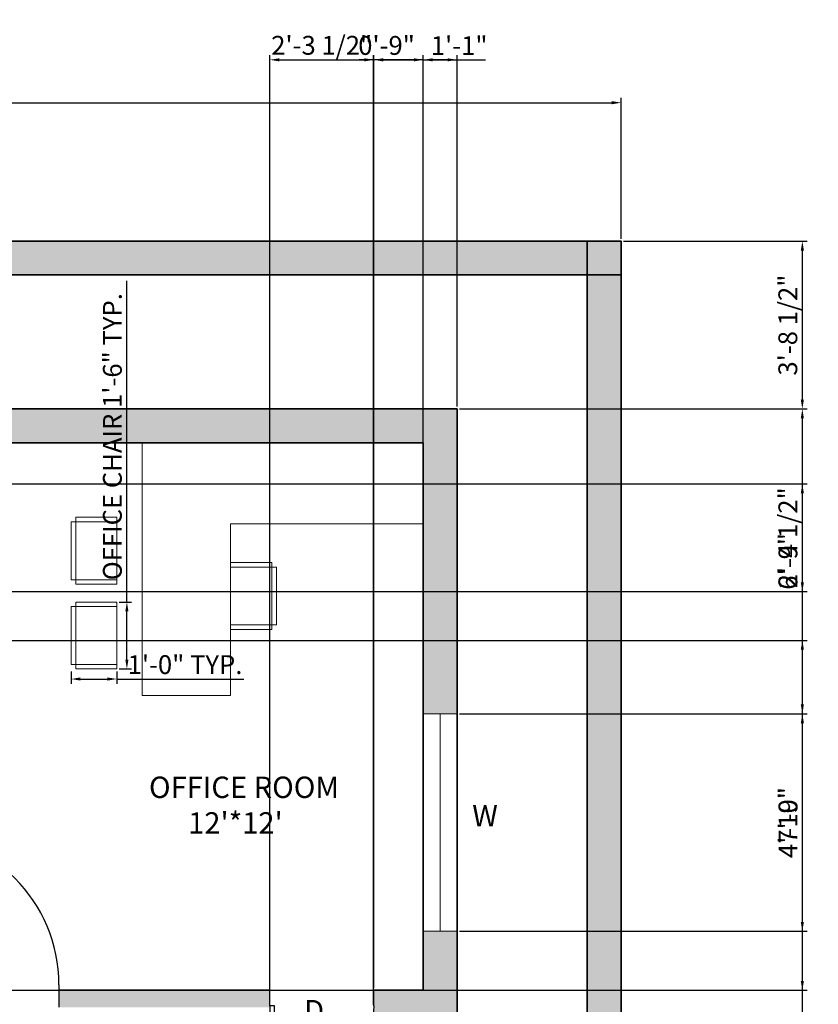
# Model space of a CAD drawing. Units: inches. Extents: x 2130 to 2621, y 981 to 1994.
# Tile 4 of 4: x 2409 to 2621, y 1732 to 1994. Entities that reach past the tile are written whole.
import ezdxf

# ---------------------------------------------------------------- set-up
doc = ezdxf.new("R2010")
doc.units = ezdxf.units.IN
for name, color, linetype, lineweight in [('A-ANNO-DIMS', 2, 'Continuous', 18), ('A-ANNO-TEXT', 10, 'Continuous', 18), ('A-AREA-IDEN', 10, 'Continuous', 18), ('A-WALL-PATT', 140, 'Continuous', 13), ('C-PROP', 7, 'Continuous', 35), ('C-PROP-PATT', 140, 'Continuous', 13), ('DOOR', 130, 'Continuous', 25), ('FUR', 190, 'Continuous', 18), ('WALL', 140, 'Continuous', 35), ('WIND', 210, 'Continuous', 18)]:
    doc.layers.add(name, color=color, linetype=linetype, lineweight=lineweight)
doc.styles.get("Standard").update_dxf_attribs({"font": 'arial.ttf'})
doc.dimstyles.new('ISO-25', dxfattribs={"dimtxt": 5, "dimasz": 2.5, "dimexe": 1.25, "dimexo": 0.625, "dimtad": 1, "dimdec": 0, "dimlunit": 4, "dimtxsty": 'Standard', "dimcen": 2.5, "dimadec": 0, "dimazin": 0, "dimtfac": 1, "dimtdec": 0, "dimtmove": 0, "dimatfit": 3, "dimfxl": 1, "dimarcsym": 0})

# ---------------------------------------------------------------- blocks, each defined once
blk = doc.blocks.new('*U2')
for p, q in [((0, 0), (0, -6)), ((40, 0), (40, -6))]:
    blk.add_line(p, q)
blk.add_lwpolyline([(0, 0), (0, 40), (1.75, 40), (1.75, 0)], close=True)
blk.add_arc((0, 0), 40, 0, 90)
blk = doc.blocks.new('*D9')
at = {"layer": 'A-ANNO-DIMS', "color": 0, "lineweight": -2, "transparency": 16777216}
for p, q in [((2188.76, 1935.64), (2188.76, 1973.06)), ((2568.76, 1935.64), (2568.76, 1973.06)), ((2191.26, 1971.81), (2566.26, 1971.81))]:
    blk.add_line(p, q, dxfattribs=at)
at = {"layer": 'A-ANNO-DIMS', "color": 0, "transparency": 16777216}
for points in [[(2191.26, 1972.23), (2191.26, 1971.39), (2188.76, 1971.81)], [(2566.26, 1972.23), (2566.26, 1971.39), (2568.76, 1971.81)]]:
    blk.add_solid(points, dxfattribs=at)
at = {"layer": 'Defpoints', "color": 0, "transparency": 16777216}
for p in [(2568.76, 1971.81), (2188.76, 1935.02), (2568.76, 1935.02)]:
    blk.add_point(p, dxfattribs=at)
at = {"layer": 'A-ANNO-DIMS', "color": 0, "transparency": 16777216, "insert": (2378.76, 1974.99), "char_height": 5, "attachment_point": 5}
blk.add_mtext('31\'-8"', dxfattribs=at)
blk = doc.blocks.new('CHAIR-OFFICE')
for p, q in [((0, 1.2), (0, 16.6)), ((0, 16.6), (1.25, 16.6)), ((1.25, 16.6), (1.25, 17.78)), ((1.25, 17.78), (12.18, 17.78)), ((12.18, 17.78), (12.18, 16.6)), ((12.18, 0), (12.18, 2.81)), ((1.25, 1.2), (0, 1.2)), ((1.25, 1.2), (1.25, 0)), ((1.25, 0), (12.18, 0))]:
    blk.add_line(p, q)
blk.add_lwpolyline([(12.18, 16.6), (1.25, 16.6), (1.25, 1.2), (12.18, 1.2)], close=True)
blk = doc.blocks.new('*D17')
at = {"layer": 'A-ANNO-DIMS', "color": 0, "lineweight": -2, "transparency": 16777216}
for p, q in [((2437.35, 1839.09), (2437.35, 1924.49)), ((2435.31, 1839.09), (2438.6, 1839.09)), ((2437.35, 1823.81), (2437.35, 1836.59)), ((2435.31, 1821.31), (2438.6, 1821.31))]:
    blk.add_line(p, q, dxfattribs=at)
at = {"layer": 'A-ANNO-DIMS', "color": 0, "transparency": 16777216}
for points in [[(2436.94, 1836.59), (2437.77, 1836.59), (2437.35, 1839.09)], [(2436.94, 1823.81), (2437.77, 1823.81), (2437.35, 1821.31)]]:
    blk.add_solid(points, dxfattribs=at)
at = {"layer": 'Defpoints', "color": 0, "transparency": 16777216}
for p in [(2434.69, 1839.09), (2437.35, 1839.09), (2434.69, 1821.31)]:
    blk.add_point(p, dxfattribs=at)
at = {"layer": 'A-ANNO-DIMS', "color": 0, "transparency": 16777216, "insert": (2434.14, 1883.04), "char_height": 5, "attachment_point": 5, "rotation": 90}
blk.add_mtext('OFFICE CHAIR 1\'-6" TYP.', dxfattribs=at)
blk = doc.blocks.new('*D18')
at = {"layer": 'A-ANNO-DIMS', "color": 0, "lineweight": -2, "transparency": 16777216}
for p, q in [((2422.5, 1820.68), (2422.5, 1817.39)), ((2425, 1818.64), (2432.19, 1818.64)), ((2434.69, 1820.68), (2434.69, 1817.39)), ((2434.69, 1818.64), (2468.44, 1818.64))]:
    blk.add_line(p, q, dxfattribs=at)
at = {"layer": 'A-ANNO-DIMS', "color": 0, "transparency": 16777216}
for points in [[(2425, 1819.06), (2425, 1818.23), (2422.5, 1818.64)], [(2432.19, 1819.06), (2432.19, 1818.23), (2434.69, 1818.64)]]:
    blk.add_solid(points, dxfattribs=at)
at = {"layer": 'Defpoints', "color": 0, "transparency": 16777216}
for p in [(2422.5, 1821.31), (2434.69, 1821.31), (2434.69, 1818.64)]:
    blk.add_point(p, dxfattribs=at)
at = {"layer": 'A-ANNO-DIMS', "color": 0, "transparency": 16777216, "insert": (2452.81, 1821.82), "char_height": 5, "attachment_point": 5}
blk.add_mtext('1\'-0" TYP.', dxfattribs=at)
blk = doc.blocks.new('*D24')
at = {"layer": 'A-ANNO-DIMS', "color": 0, "lineweight": -2, "transparency": 16777216}
for p, q in [((2525.79, 1890.41), (2618.19, 1890.41)), ((2616.94, 1355.91), (2616.94, 1887.91)), ((2525.79, 1353.41), (2618.19, 1353.41))]:
    blk.add_line(p, q, dxfattribs=at)
at = {"layer": 'A-ANNO-DIMS', "color": 0, "transparency": 16777216}
for points in [[(2616.52, 1887.91), (2617.35, 1887.91), (2616.94, 1890.41)], [(2616.52, 1355.91), (2617.35, 1355.91), (2616.94, 1353.41)]]:
    blk.add_solid(points, dxfattribs=at)
at = {"layer": 'Defpoints', "color": 0, "transparency": 16777216}
for p in [(2525.16, 1890.41), (2616.94, 1890.41), (2525.16, 1353.41)]:
    blk.add_point(p, dxfattribs=at)
at = {"layer": 'A-ANNO-DIMS', "color": 0, "transparency": 16777216, "insert": (2613.76, 1621.91), "char_height": 5, "attachment_point": 5, "rotation": 90}
blk.add_mtext('44\'-9"', dxfattribs=at)
blk = doc.blocks.new('*D26')
at = {"layer": 'A-ANNO-DIMS', "color": 0, "lineweight": -2, "transparency": 16777216}
for p, q in [((2569.38, 1935.02), (2618.19, 1935.02)), ((2616.94, 1892.91), (2616.94, 1932.52)), ((2525.79, 1890.41), (2618.19, 1890.41))]:
    blk.add_line(p, q, dxfattribs=at)
at = {"layer": 'A-ANNO-DIMS', "color": 0, "transparency": 16777216}
for points in [[(2616.52, 1932.52), (2617.35, 1932.52), (2616.94, 1935.02)], [(2616.52, 1892.91), (2617.35, 1892.91), (2616.94, 1890.41)]]:
    blk.add_solid(points, dxfattribs=at)
at = {"layer": 'Defpoints', "color": 0, "transparency": 16777216}
for p in [(2568.76, 1935.02), (2616.94, 1935.02), (2525.16, 1890.41)]:
    blk.add_point(p, dxfattribs=at)
at = {"layer": 'A-ANNO-DIMS', "color": 0, "transparency": 16777216, "insert": (2613.72, 1912.71), "char_height": 5, "attachment_point": 5, "rotation": 90}
blk.add_mtext('3\'-8 1/2"', dxfattribs=at)
blk = doc.blocks.new('*D29')
at = {"layer": 'A-ANNO-DIMS', "color": 0, "lineweight": -2, "transparency": 16777216}
for p, q in [((2368.29, 1828.91), (2618.19, 1828.91)), ((2616.94, 1738.41), (2616.94, 1826.41)), ((2368.29, 1735.91), (2618.19, 1735.91))]:
    blk.add_line(p, q, dxfattribs=at)
at = {"layer": 'A-ANNO-DIMS', "color": 0, "transparency": 16777216}
for points in [[(2616.52, 1826.41), (2617.35, 1826.41), (2616.94, 1828.91)], [(2616.52, 1738.41), (2617.35, 1738.41), (2616.94, 1735.91)]]:
    blk.add_solid(points, dxfattribs=at)
at = {"layer": 'Defpoints', "color": 0, "transparency": 16777216}
for p in [(2367.66, 1828.91), (2616.94, 1828.91), (2367.66, 1735.91)]:
    blk.add_point(p, dxfattribs=at)
at = {"layer": 'A-ANNO-DIMS', "color": 0, "transparency": 16777216, "insert": (2613.76, 1782.41), "char_height": 5, "attachment_point": 5, "rotation": 90}
blk.add_mtext('7\'-9"', dxfattribs=at)
blk = doc.blocks.new('*D37')
at = {"layer": 'A-ANNO-DIMS', "color": 0, "lineweight": -2, "transparency": 16777216}
for p, q in [((2475.37, 1732.39), (2475.37, 1984.45)), ((2502.94, 1732.04), (2502.94, 1984.45)), ((2477.87, 1983.2), (2500.44, 1983.2))]:
    blk.add_line(p, q, dxfattribs=at)
at = {"layer": 'A-ANNO-DIMS', "color": 0, "transparency": 16777216}
for points in [[(2477.87, 1983.61), (2477.87, 1982.78), (2475.37, 1983.2)], [(2500.44, 1983.61), (2500.44, 1982.78), (2502.94, 1983.2)]]:
    blk.add_solid(points, dxfattribs=at)
at = {"layer": 'Defpoints', "color": 0, "transparency": 16777216}
for p in [(2502.94, 1983.2), (2475.37, 1731.77), (2502.94, 1731.41)]:
    blk.add_point(p, dxfattribs=at)
at = {"layer": 'A-ANNO-DIMS', "color": 0, "transparency": 16777216, "insert": (2489.15, 1986.41), "char_height": 5, "attachment_point": 5}
blk.add_mtext('2\'-3 1/2"', dxfattribs=at)
blk = doc.blocks.new('*D39')
at = {"layer": 'A-ANNO-DIMS', "color": 0, "lineweight": -2, "transparency": 16777216}
for p, q in [((2525.79, 1809.41), (2618.19, 1809.41)), ((2616.94, 1754.09), (2616.94, 1806.91)), ((2525.79, 1751.59), (2618.19, 1751.59))]:
    blk.add_line(p, q, dxfattribs=at)
at = {"layer": 'A-ANNO-DIMS', "color": 0, "transparency": 16777216}
for points in [[(2616.52, 1806.91), (2617.35, 1806.91), (2616.94, 1809.41)], [(2616.52, 1754.09), (2617.35, 1754.09), (2616.94, 1751.59)]]:
    blk.add_solid(points, dxfattribs=at)
at = {"layer": 'Defpoints', "color": 0, "transparency": 16777216}
for p in [(2525.16, 1809.41), (2616.94, 1809.41), (2525.16, 1751.59)]:
    blk.add_point(p, dxfattribs=at)
at = {"layer": 'A-ANNO-DIMS', "color": 0, "transparency": 16777216, "insert": (2613.76, 1780.5), "char_height": 5, "attachment_point": 5, "rotation": 90}
blk.add_mtext('4\'-10"', dxfattribs=at)
blk = doc.blocks.new('*D40')
at = {"layer": 'A-ANNO-DIMS', "color": 0, "lineweight": -2, "transparency": 16777216}
for p, q in [((2525.79, 1890.41), (2618.19, 1890.41)), ((2616.94, 1811.91), (2616.94, 1887.91)), ((2525.79, 1809.41), (2618.19, 1809.41))]:
    blk.add_line(p, q, dxfattribs=at)
at = {"layer": 'A-ANNO-DIMS', "color": 0, "transparency": 16777216}
for points in [[(2616.52, 1887.91), (2617.35, 1887.91), (2616.94, 1890.41)], [(2616.52, 1811.91), (2617.35, 1811.91), (2616.94, 1809.41)]]:
    blk.add_solid(points, dxfattribs=at)
at = {"layer": 'Defpoints', "color": 0, "transparency": 16777216}
for p in [(2525.16, 1890.41), (2616.94, 1890.41), (2525.16, 1809.41)]:
    blk.add_point(p, dxfattribs=at)
at = {"layer": 'A-ANNO-DIMS', "color": 0, "transparency": 16777216, "insert": (2613.76, 1849.91), "char_height": 5, "attachment_point": 5, "rotation": 90}
blk.add_mtext('6\'-9"', dxfattribs=at)
blk = doc.blocks.new('*D43')
at = {"layer": 'A-ANNO-DIMS', "color": 0, "lineweight": -2, "transparency": 16777216}
for p, q in [((2231.79, 1870.49), (2618.19, 1870.49)), ((2616.94, 1844.36), (2616.94, 1867.99)), ((2231.79, 1841.86), (2618.19, 1841.86))]:
    blk.add_line(p, q, dxfattribs=at)
at = {"layer": 'A-ANNO-DIMS', "color": 0, "transparency": 16777216}
for points in [[(2616.52, 1867.99), (2617.35, 1867.99), (2616.94, 1870.49)], [(2616.52, 1844.36), (2617.35, 1844.36), (2616.94, 1841.86)]]:
    blk.add_solid(points, dxfattribs=at)
at = {"layer": 'Defpoints', "color": 0, "transparency": 16777216}
for p in [(2231.16, 1870.49), (2616.94, 1870.49), (2231.16, 1841.86)]:
    blk.add_point(p, dxfattribs=at)
at = {"layer": 'A-ANNO-DIMS', "color": 0, "transparency": 16777216, "insert": (2613.73, 1856.18), "char_height": 5, "attachment_point": 5, "rotation": 90}
blk.add_mtext('2\'-4 1/2"', dxfattribs=at)
blk = doc.blocks.new('*D49')
at = {"layer": 'A-ANNO-DIMS', "color": 0, "lineweight": -2, "transparency": 16777216}
for p, q in [((2516.16, 1882.04), (2516.16, 1984.45)), ((2525.16, 1891.04), (2525.16, 1984.45)), ((2516.16, 1983.2), (2499.12, 1983.2)), ((2522.66, 1983.2), (2518.66, 1983.2))]:
    blk.add_line(p, q, dxfattribs=at)
at = {"layer": 'A-ANNO-DIMS', "color": 0, "transparency": 16777216}
for points in [[(2518.66, 1983.61), (2518.66, 1982.78), (2516.16, 1983.2)], [(2522.66, 1983.61), (2522.66, 1982.78), (2525.16, 1983.2)]]:
    blk.add_solid(points, dxfattribs=at)
at = {"layer": 'Defpoints', "color": 0, "transparency": 16777216}
for p in [(2516.16, 1983.2), (2525.16, 1890.41), (2516.16, 1881.41)]:
    blk.add_point(p, dxfattribs=at)
at = {"layer": 'A-ANNO-DIMS', "color": 0, "transparency": 16777216, "insert": (2506.39, 1986.37), "char_height": 5, "attachment_point": 5}
blk.add_mtext('0\'-9"', dxfattribs=at)
blk = doc.blocks.new('*D53')
at = {"layer": 'A-ANNO-DIMS', "color": 0, "lineweight": -2, "transparency": 16777216}
for p, q in [((2503, 1736.54), (2503, 1984.45)), ((2516.16, 1736.54), (2516.16, 1984.45)), ((2505.5, 1983.2), (2513.66, 1983.2)), ((2516.16, 1983.2), (2532.73, 1983.2))]:
    blk.add_line(p, q, dxfattribs=at)
at = {"layer": 'A-ANNO-DIMS', "color": 0, "transparency": 16777216}
for points in [[(2505.5, 1983.61), (2505.5, 1982.78), (2503, 1983.2)], [(2513.66, 1983.61), (2513.66, 1982.78), (2516.16, 1983.2)]]:
    blk.add_solid(points, dxfattribs=at)
at = {"layer": 'Defpoints', "color": 0, "transparency": 16777216}
for p in [(2516.16, 1983.2), (2503, 1735.91), (2516.16, 1735.91)]:
    blk.add_point(p, dxfattribs=at)
at = {"layer": 'A-ANNO-DIMS', "color": 0, "transparency": 16777216, "insert": (2525.7, 1986.33), "char_height": 5, "attachment_point": 5}
blk.add_mtext('1\'-1"', dxfattribs=at)

msp = doc.modelspace()

# ---------------------------------------------------------------- hatches: boundary and pattern name
at = {"layer": 'A-WALL-PATT'}
h = msp.add_hatch(color=256, dxfattribs=at)
h.dxf.hatch_style = 1
h.paths.add_polyline_path([(2272.17, 1886.91), (2272.17, 1890.41), (2222.16, 1890.41), (2222.16, 1870.49), (2231.16, 1870.49), (2231.16, 1881.41), (2272.82, 1881.41, -0.059514)])
h.paths.add_polyline_path([(2231.16, 1828.91), (2301.66, 1828.91), (2301.66, 1881.41), (2297.16, 1881.41), (2297.16, 1833.41), (2265.07, 1833.41), (2231.16, 1833.41), (2231.16, 1841.86), (2222.16, 1841.86), (2222.16, 1828.91), (2222.16, 1790.61), (2228.16, 1790.61, -0.01877), (2231.16, 1790.5)])
h.paths.add_polyline_path([(2303.95, 1886.91), (2303.95, 1890.41), (2301.66, 1890.41), (2295.51, 1890.41), (2295.51, 1886.91), (2295.51, 1881.41), (2297.16, 1881.41), (2301.66, 1881.41), (2303.95, 1881.41)])
h.paths.add_polyline_path([(2525.16, 1890.41), (2372.16, 1890.41), (2327.29, 1890.41), (2327.29, 1886.91, -0.059514), (2326.63, 1881.41), (2367.66, 1881.41), (2367.66, 1833.41), (2361.98, 1833.41), (2361.98, 1828.91), (2367.66, 1828.91), (2367.66, 1735.91), (2372.16, 1735.91), (2372.16, 1828.91), (2372.16, 1881.41), (2516.16, 1881.41), (2516.16, 1859.91), (2516.16, 1809.41), (2525.16, 1809.41)])
h.paths.add_polyline_path([(2475.37, 1735.91), (2419.27, 1735.91), (2419.27, 1731.41), (2475.37, 1731.41), (2475.37, 1731.77)])
h.paths.add_polyline_path([(2525.16, 1751.59), (2516.16, 1751.59), (2516.16, 1737.41), (2516.16, 1735.91), (2503, 1735.91), (2503, 1731.77, -0.030428), (2502.8, 1728.41), (2516.16, 1728.41), (2516.16, 1714.24), (2525.16, 1714.24), (2525.16, 1728.41)])
h.paths.add_polyline_path([(2379.27, 1735.91), (2231.16, 1735.91), (2231.16, 1731.41), (2379.27, 1731.41)])
h.paths.add_polyline_path([(2231.16, 1728.41), (2231.16, 1735.91), (2231.16, 1750.61), (2228.16, 1750.61), (2222.16, 1750.61), (2222.16, 1728.41), (2222.16, 1674.58), (2231.16, 1674.58)])
h.paths.add_polyline_path([(2516.16, 1584.41), (2462.16, 1584.41), (2403.94, 1584.41), (2403.94, 1575.41), (2404.07, 1575.41), (2453.16, 1575.41), (2516.16, 1575.41)], flags=17)
h.paths.add_polyline_path([(2516.16, 1584.41), (2462.16, 1584.41), (2403.94, 1584.41), (2403.94, 1575.41), (2453.16, 1575.41), (2516.16, 1575.41)], flags=17)
h.paths.add_polyline_path([(2318.23, 1584.41), (2231.16, 1584.41), (2231.16, 1575.41), (2318.23, 1575.41)])
h = msp.add_hatch(color=256, dxfattribs=at)
h.dxf.hatch_style = 1
h.paths.add_polyline_path([(2231.16, 1595.8), (2222.16, 1595.8), (2222.16, 1571.6), (2225.81, 1571.6), (2231.16, 1571.6)])
h.paths.add_polyline_path([(2313.28, 1362.41), (2237.26, 1362.41), (2231.16, 1362.41), (2231.16, 1404.41), (2231.16, 1474.85), (2231.16, 1547.86, -0.05547), (2225.81, 1547.27), (2222.16, 1547.27), (2222.16, 1425.41), (2222.16, 1353.41), (2313.28, 1353.41)])
h.paths.add_polyline_path([(2393.01, 1195.09), (2434.46, 1195.09), (2434.46, 1216.28), (2393.01, 1216.28)], flags=9)
h.paths.add_polyline_path([(2245.08, 1335), (2303.47, 1335), (2303.47, 1346.7), (2245.08, 1346.7)], flags=9)
h.paths.add_polyline_path([(2458.81, 1338.38), (2517.21, 1338.38), (2517.21, 1350.09), (2458.81, 1350.09)], flags=9)
h.paths.add_polyline_path([(2232.7, 1530.42), (2263.31, 1530.42), (2263.31, 1551.62), (2232.7, 1551.62)], flags=9)
h.paths.add_polyline_path([(2332.94, 1458.61), (2399.05, 1458.61), (2399.05, 1489.37), (2332.94, 1489.37)], flags=9)
h.paths.add_polyline_path([(2475.66, 1607.66), (2507.9, 1607.66), (2507.9, 1628.85), (2475.66, 1628.85)], flags=9)
h.paths.add_polyline_path([(2486.7, 1688.97), (2517.32, 1688.97), (2517.32, 1710.17), (2486.7, 1710.17)], flags=9)
h.paths.add_polyline_path([(2333.88, 1649.81), (2375.07, 1649.81), (2375.07, 1671), (2333.88, 1671)], flags=9)
h.paths.add_polyline_path([(2441.42, 1774.34), (2500.24, 1774.34), (2500.24, 1795.53), (2441.42, 1795.53)], flags=9)
h.paths.add_polyline_path([(2332.74, 1857.16), (2363.5, 1857.16), (2363.5, 1878.35), (2332.74, 1878.35)], flags=9)
h.paths.add_polyline_path([(2244.84, 1853.21), (2275.6, 1853.21), (2275.6, 1874.4), (2244.84, 1874.4)], flags=9)
at = {"layer": 'C-PROP-PATT'}
h = msp.add_hatch(color=256, dxfattribs=at)
h.dxf.hatch_style = 1
h.paths.add_polyline_path([(2559.76, 1935.02), (2197.76, 1935.02), (2197.76, 1926.02), (2559.76, 1926.02)])
h.paths.add_polyline_path([(2197.76, 1935.02), (2188.76, 1935.02), (2188.76, 1077.41), (2197.76, 1077.41)])
h.paths.add_polyline_path([(2568.76, 1926.02), (2559.76, 1926.02), (2559.76, 1077.41), (2568.76, 1077.41)])
h.paths.add_polyline_path([(2568.76, 1935.02), (2559.76, 1935.02), (2559.76, 1926.02), (2568.76, 1926.02)])

# ---------------------------------------------------------------- linework, layer by layer
at = {"layer": 'C-PROP'}
for p, q in [((2188.76, 1935.02), (2568.76, 1935.02)), ((2568.76, 1935.02), (2568.76, 1077.41)), ((2197.76, 1926.02), (2559.76, 1926.02)), ((2559.76, 1926.02), (2559.76, 1086.41))]:
    msp.add_line(p, q, dxfattribs=at)
for points in [[(2197.76, 1926.02), (2568.76, 1926.02), (2568.76, 1935.02), (2197.76, 1935.02)], [(2559.76, 1077.41), (2568.76, 1077.41), (2568.76, 1935.02), (2559.76, 1935.02)]]:
    msp.add_lwpolyline(points, close=True, dxfattribs=at)
at = {"layer": 'FUR'}
for p, q in [((2475.85, 1849.6), (2464.92, 1849.6)), ((2475.85, 1848.4), (2475.85, 1849.6)), ((2475.85, 1848.4), (2477.11, 1848.4)), ((2477.11, 1848.4), (2477.11, 1833)), ((2464.92, 1846), (2464.92, 1843.19)), ((2475.85, 1831.82), (2464.92, 1831.82)), ((2477.11, 1833), (2475.85, 1833)), ((2475.85, 1833), (2475.85, 1831.82)), ((2464.92, 1828.22), (2464.92, 1829.4))]:
    msp.add_line(p, q, dxfattribs=at)
for points in [[(2464.92, 1859.91), (2516.16, 1859.91), (2516.16, 1881.41), (2441.43, 1881.41), (2441.43, 1859.91)], [(2464.92, 1859.91), (2464.92, 1814.29), (2441.43, 1814.29), (2441.43, 1881.41), (2464.92, 1881.41)]]:
    msp.add_lwpolyline(points, dxfattribs=at)
msp.add_lwpolyline([(2464.92, 1833), (2475.85, 1833), (2475.85, 1848.4), (2464.92, 1848.4)], close=True, dxfattribs=at)
at = {"layer": 'WALL'}
for p, q in [((2372.16, 1890.41), (2525.16, 1890.41)), ((2525.16, 1890.41), (2525.16, 1728.41)), ((2372.16, 1881.41), (2516.16, 1881.41)), ((2516.16, 1881.41), (2516.16, 1737.41)), ((2516.16, 1735.91), (2516.16, 1739.53)), ((2419.27, 1735.91), (2475.37, 1735.91)), ((2503, 1735.91), (2516.16, 1735.91))]:
    msp.add_line(p, q, dxfattribs=at)
at = {"layer": 'WIND'}
msp.add_line((2520.66, 1751.59), (2520.66, 1809.41), dxfattribs=at)
msp.add_lwpolyline([(2516.16, 1751.59), (2525.16, 1751.59), (2525.16, 1809.41), (2516.16, 1809.41)], close=True, dxfattribs=at)

# ---------------------------------------------------------------- block references
at = {"layer": 'DOOR'}
msp.add_blockref('*U2', (2379.27, 1737.41), dxfattribs=at)
at = {"layer": 'DOOR', "xscale": -0.6909314595712287, "yscale": 0.6909314595712287, "zscale": 0.6909314595712287, "rotation": 180}
msp.add_blockref('*U2', (2475.37, 1731.77), dxfattribs=at)
at = {"layer": 'FUR'}
for p in [(2422.5, 1843.84), (2422.5, 1821.31)]:
    msp.add_blockref('CHAIR-OFFICE', p, dxfattribs=at)

# ---------------------------------------------------------------- texts
at = {"layer": 'A-ANNO-TEXT', "char_height": 5.68, "attachment_point": 1}
for s, insert in [('W', (2529.17, 1785.14)), ('D', (2484.47, 1733.34))]:
    msp.add_mtext_dynamic_manual_height_columns(s, width=39.9661, gutter_width=28.4, heights=[0], dxfattribs=dict(at, insert=insert))
at = {"layer": 'A-AREA-IDEN', "insert": (2443.23, 1792.71), "char_height": 5.6797, "attachment_point": 1}
msp.add_mtext_dynamic_manual_height_columns("OFFICE ROOM\\P      12'*12'", width=62.1593, gutter_width=28.4, heights=[0], dxfattribs=at)

# ---------------------------------------------------------------- dimensions: what is measured, and where the dimension line sits
at = {"layer": 'A-ANNO-DIMS'}
for base, p1, p2, override, picture, middle in [((2502.94, 1983.2), (2475.37, 1731.77), (2502.94, 1731.41), {"dimdec": 1, "dimlfac": 1, "dimrnd": 0, "dimzin": 1, "dimdsep": 46, "dimlunit": 4, "dimfrac": 2}, '*D37', (2489.15, 1986.41)), ((2516.16, 1983.2), (2525.16, 1890.41), (2516.16, 1881.41), {"dimdec": 1, "dimlfac": 1, "dimrnd": 0, "dimzin": 1, "dimdsep": 46, "dimlunit": 4, "dimfrac": 2}, '*D49', (2506.39, 1986.37)), ((2516.16, 1983.2), (2503, 1735.91), (2516.16, 1735.91), {"dimdec": 1, "dimlfac": 1, "dimrnd": 0, "dimzin": 1, "dimdsep": 46, "dimlunit": 4, "dimfrac": 2}, '*D53', (2525.7, 1986.33)), ((2568.76, 1971.81), (2188.76, 1935.02), (2568.76, 1935.02), {"dimclrd": 0, "dimclre": 0, "dimclrt": 0}, '*D9', (2378.76, 1974.99))]:
    dim = msp.add_linear_dim(base=base, p1=p1, p2=p2, dimstyle='ISO-25', override=override, dxfattribs=at)
    dim.commit()
    dim.dimension.update_dxf_attribs({"geometry": picture, "text_midpoint": middle})
for base, p1, p2, picture, middle in [((2616.94, 1935.02), (2525.16, 1890.41), (2568.76, 1935.02), '*D26', (2613.72, 1912.71)), ((2616.94, 1890.41), (2525.16, 1353.41), (2525.16, 1890.41), '*D24', (2613.76, 1621.91)), ((2616.94, 1890.41), (2525.16, 1809.41), (2525.16, 1890.41), '*D40', (2613.76, 1849.91)), ((2616.94, 1870.49), (2231.16, 1841.86), (2231.16, 1870.49), '*D43', (2613.73, 1856.18)), ((2616.94, 1828.91), (2367.66, 1735.91), (2367.66, 1828.91), '*D29', (2613.76, 1782.41)), ((2616.94, 1809.41), (2525.16, 1751.59), (2525.16, 1809.41), '*D39', (2613.76, 1780.5))]:
    dim = msp.add_linear_dim(base=base, p1=p1, p2=p2, angle=90, dimstyle='ISO-25', override={"dimdec": 1, "dimlfac": 1, "dimrnd": 0, "dimzin": 1, "dimdsep": 46, "dimlunit": 4, "dimfrac": 2}, dxfattribs=at)
    dim.commit()
    dim.dimension.update_dxf_attribs({"geometry": picture, "text_midpoint": middle})
dim = msp.add_linear_dim(base=(2437.35, 1839.09), p1=(2434.69, 1821.31), p2=(2434.69, 1839.09), angle=90, text='OFFICE CHAIR <> TYP.', dimstyle='ISO-25', override={"dimdec": 1, "dimlfac": 1, "dimrnd": 0, "dimzin": 1, "dimdsep": 46, "dimlunit": 4, "dimfrac": 2}, dxfattribs=at)
dim.commit()
dim.dimension.update_dxf_attribs({"geometry": '*D17', "text_midpoint": (2434.14, 1883.04)})
dim = msp.add_linear_dim(base=(2434.69, 1818.64), p1=(2422.5, 1821.31), p2=(2434.69, 1821.31), text='<> TYP.', dimstyle='ISO-25', override={"dimdec": 1, "dimlfac": 1, "dimrnd": 0, "dimzin": 1, "dimdsep": 46, "dimlunit": 4, "dimfrac": 2}, dxfattribs=at)
dim.commit()
dim.dimension.update_dxf_attribs({"geometry": '*D18', "text_midpoint": (2452.81, 1821.82)})

doc.saveas('drawing.dxf')
